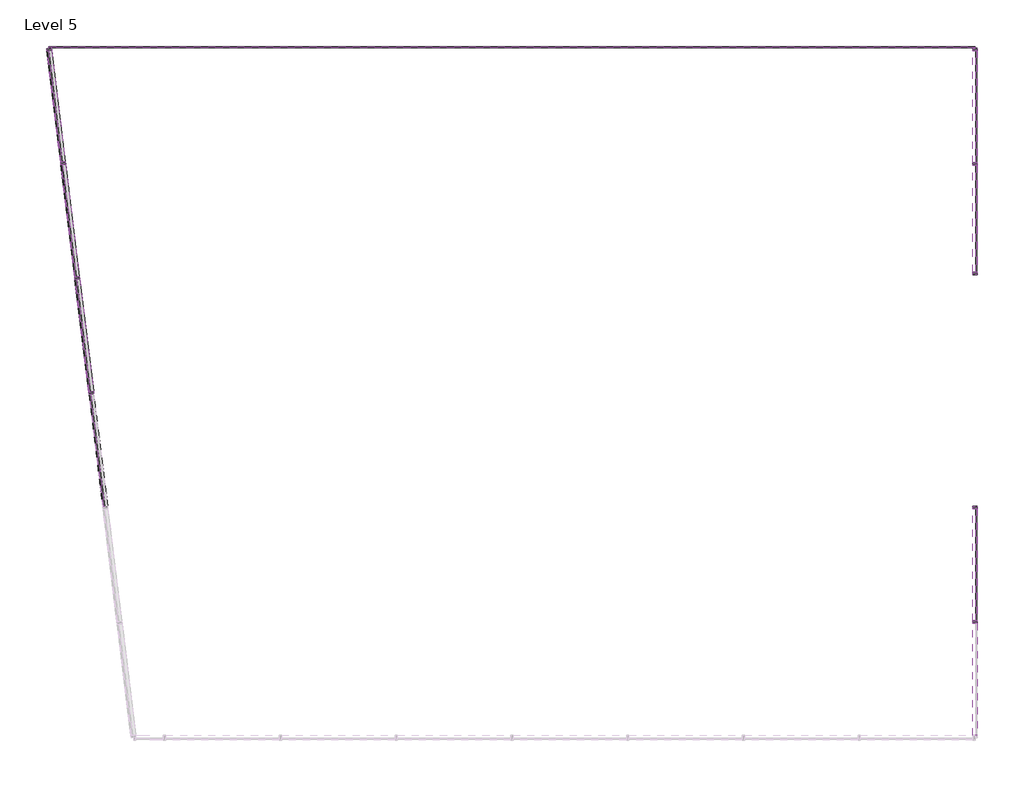
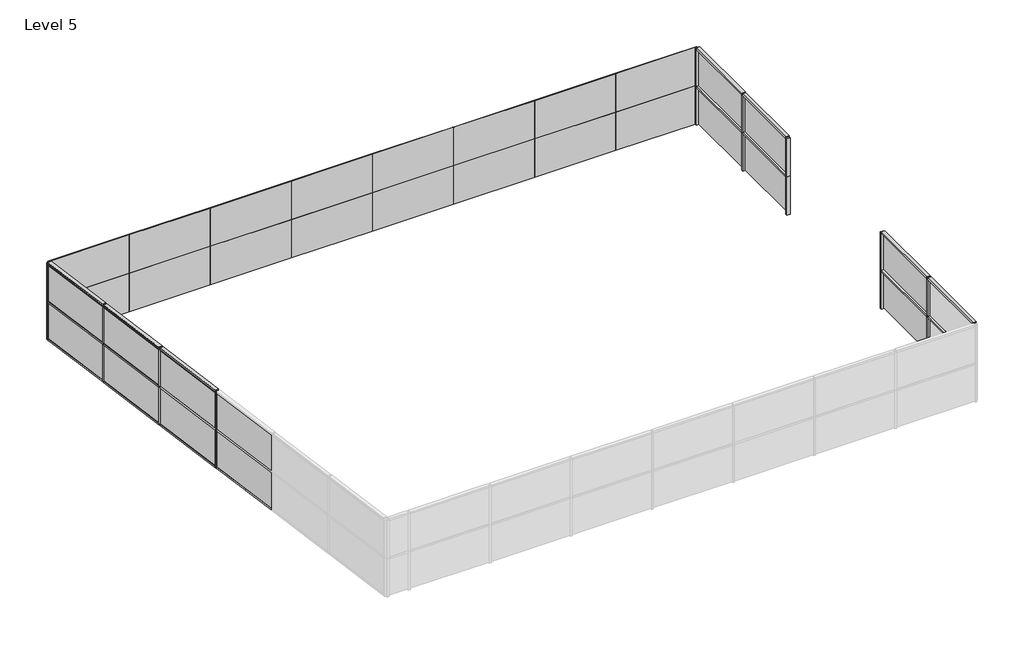
# One storey, part 2 of 2: 50 members, 38 plates.
"""IFC4 building model written with IfcOpenShell, lengths in millimetres."""

from ifc_helpers import new_model, si_unit, origin, place, context, project, spatial, transform, mapped, element, save
from components import member_71c27fd2, member_daa7a266, member_82905deb, member_19d0a4ec, member_8cef0660, member_db480205, member_4491d118, member_46bdb8c2, system_panel_glazed_1e57f9bb, system_panel_glazed_37f15d2e, system_panel_glazed_3620f98e, system_panel_glazed_e46d4b42, system_panel_glazed_2a6c68b7, system_panel_glazed_d483336f

model = new_model("IFC4")

# Units and contexts
model_context = context("Model", 3, world=origin())
ifc_project = project(units=[si_unit("LENGTHUNIT", "METRE", prefix="MILLI")], contexts=[model_context])

# Site, building, storey
site = spatial("IfcSite", under=ifc_project)
building = spatial("IfcBuilding", under=site)
storey = spatial("IfcBuildingStorey", under=building, Name="Level 5", Elevation=12192.0)

# Members
placement = place(None, origin())
member_shape = member_71c27fd2(model_context)
element("IfcMember", 1, ObjectType="Rectangular Mullion : 2.5\" x 5\" rectangular", at=placement, inside=storey, context=model_context, shape_type="MappedRepresentation", body=[
    mapped(member_shape, transform((-10473.7456604, 11109.5209701, 12192.0), x_axis=(0.0, 0.0, -1.0), y_axis=(-0.9925461516413222, -0.12186934340514603, 0.0), z_axis=(-0.12186934340514603, 0.9925461516413222, 0.0))),
])
member_2_shape = member_daa7a266(model_context)
element("IfcMember", 2, ObjectType="Rectangular Mullion : 2.5\" x 5\" rectangular", at=placement, inside=storey, context=model_context, shape_type="MappedRepresentation", body=[
    mapped(member_2_shape, transform((-10113.8959567, 8178.7803212, 15240.0), x_axis=(0.0, 0.0, 1.0), y_axis=(-0.9925461516413222, -0.12186934340514625, 0.0), z_axis=(0.12186934340514625, -0.9925461516413222, 0.0))),
])
member_3_shape = member_82905deb(model_context)
element("IfcMember", 3, ObjectType="Rectangular Mullion : 2.5\" x 5\" rectangular", at=placement, inside=storey, context=model_context, shape_type="MappedRepresentation", body=[
    mapped(member_3_shape, transform((-9367.1110876, 2096.7056405, 15240.0), x_axis=(-0.1218693434051459, 0.9925461516413222, 0.0), y_axis=(-0.9925461516413222, -0.1218693434051459, 0.0), z_axis=(0.0, 0.0, 1.0))),
])
element("IfcMember", 4, ObjectType="Rectangular Mullion : 2.5\" x 5\" rectangular", at=placement, inside=storey, context=model_context, shape_type="MappedRepresentation", body=[
    mapped(member_3_shape, transform((-9738.5688463, 5121.9863107, 15240.0), x_axis=(-0.1218693434051459, 0.9925461516413222, 0.0), y_axis=(-0.9925461516413222, -0.1218693434051459, 0.0), z_axis=(0.0, 0.0, 1.0))),
])
element("IfcMember", 5, ObjectType="Rectangular Mullion : 2.5\" x 5\" rectangular", at=placement, inside=storey, context=model_context, shape_type="MappedRepresentation", body=[
    mapped(member_3_shape, transform((-10110.026605, 8147.2669809, 15240.0), x_axis=(-0.1218693434051459, 0.9925461516413222, 0.0), y_axis=(-0.9925461516413222, -0.1218693434051459, 0.0), z_axis=(0.0, 0.0, 1.0))),
])
member_4_shape = member_19d0a4ec(model_context)
element("IfcMember", 6, ObjectType="Rectangular Mullion : 2.5\" x 5\" rectangular", at=placement, inside=storey, context=model_context, shape_type="MappedRepresentation", body=[
    mapped(member_4_shape, transform((-10113.8959567, 8178.7803212, 13716.0), x_axis=(0.0, 0.0, 1.0), y_axis=(-0.9925461516413222, -0.12186934340514609, 0.0), z_axis=(0.12186934340514609, -0.9925461516413222, 0.0))),
])
element("IfcMember", 7, ObjectType="Rectangular Mullion : 2.5\" x 5\" rectangular", at=placement, inside=storey, context=model_context, shape_type="MappedRepresentation", body=[
    mapped(member_4_shape, transform((-10113.8959567, 8178.7803212, 15240.0), x_axis=(0.0, 0.0, 1.0), y_axis=(-0.9925461516413223, -0.1218693434051454, 0.0), z_axis=(0.1218693434051454, -0.9925461516413223, 0.0))),
])
element("IfcMember", 8, ObjectType="Rectangular Mullion : 2.5\" x 5\" rectangular", at=placement, inside=storey, context=model_context, shape_type="MappedRepresentation", body=[
    mapped(member_4_shape, transform((-10113.8959567, 8178.7803212, 13716.0), x_axis=(0.0, 0.0, 1.0), y_axis=(-0.9925461516413223, -0.1218693434051456, 0.0), z_axis=(0.12186934340514559, -0.9925461516413222, 0.0))),
])
element("IfcMember", 9, ObjectType="Rectangular Mullion : 2.5\" x 5\" rectangular", at=placement, inside=storey, context=model_context, shape_type="MappedRepresentation", body=[
    mapped(member_4_shape, transform((13902.5156363, -946.6363705, 13716.0), x_axis=(0.0, 0.0, 1.0), y_axis=(1.0, 0.0, 0.0), z_axis=(0.0, 1.0, 0.0))),
])
element("IfcMember", 10, ObjectType="Rectangular Mullion : 2.5\" x 5\" rectangular", at=placement, inside=storey, context=model_context, shape_type="MappedRepresentation", body=[
    mapped(member_4_shape, transform((13902.5156363, -3962.8863708, 13716.0), x_axis=(0.0, 0.0, 1.0), y_axis=(1.0, 0.0, 0.0), z_axis=(0.0, 1.0, 0.0))),
])
element("IfcMember", 11, ObjectType="Rectangular Mullion : 2.5\" x 5\" rectangular", at=placement, inside=storey, context=model_context, shape_type="MappedRepresentation", body=[
    mapped(member_4_shape, transform((13902.5156363, -946.6363705, 15240.0), x_axis=(0.0, 0.0, 1.0), y_axis=(1.0, 0.0, 0.0), z_axis=(0.0, 1.0, 0.0))),
])
element("IfcMember", 12, ObjectType="Rectangular Mullion : 2.5\" x 5\" rectangular", at=placement, inside=storey, context=model_context, shape_type="MappedRepresentation", body=[
    mapped(member_4_shape, transform((13902.5156363, -3962.8863708, 15240.0), x_axis=(0.0, 0.0, 1.0), y_axis=(1.0, 0.0, 0.0), z_axis=(0.0, 1.0, 0.0))),
])
element("IfcMember", 13, ObjectType="Rectangular Mullion : 2.5\" x 5\" rectangular", at=placement, inside=storey, context=model_context, shape_type="MappedRepresentation", body=[
    mapped(member_4_shape, transform((13902.5156363, 11109.0476508, 13716.0), x_axis=(0.0, 0.0, 1.0), y_axis=(1.0, 0.0, 0.0), z_axis=(0.0, 1.0, 0.0))),
])
element("IfcMember", 14, ObjectType="Rectangular Mullion : 2.5\" x 5\" rectangular", at=placement, inside=storey, context=model_context, shape_type="MappedRepresentation", body=[
    mapped(member_4_shape, transform((13902.5156363, 11109.0476508, 15240.0), x_axis=(0.0, 0.0, 1.0), y_axis=(1.0, 0.0, 0.0), z_axis=(0.0, 1.0, 0.0))),
])
member_5_shape = member_8cef0660(model_context)
element("IfcMember", 15, ObjectType="Rectangular Mullion : 2.5\" x 5\" rectangular", at=placement, inside=storey, context=model_context, shape_type="MappedRepresentation", body=[
    mapped(member_5_shape, transform((-9370.9804393, 2128.2189808, 13716.0), x_axis=(0.0, 0.0, 1.0), y_axis=(-0.9925461516413222, -0.12186934340514592, 0.0), z_axis=(0.12186934340514592, -0.9925461516413222, 0.0))),
])
element("IfcMember", 16, ObjectType="Rectangular Mullion : 2.5\" x 5\" rectangular", at=placement, inside=storey, context=model_context, shape_type="MappedRepresentation", body=[
    mapped(member_5_shape, transform((-9742.438198, 5153.499651, 13716.0), x_axis=(0.0, 0.0, 1.0), y_axis=(-0.9925461516413222, -0.1218693434051457, 0.0), z_axis=(0.1218693434051457, -0.9925461516413222, 0.0))),
])
element("IfcMember", 17, ObjectType="Rectangular Mullion : 2.5\" x 5\" rectangular", at=placement, inside=storey, context=model_context, shape_type="MappedRepresentation", body=[
    mapped(member_5_shape, transform((-9370.9804393, 2128.2189808, 15240.0), x_axis=(0.0, 0.0, 1.0), y_axis=(-0.9925461516413222, -0.12186934340514592, 0.0), z_axis=(0.12186934340514592, -0.9925461516413222, 0.0))),
])
element("IfcMember", 18, ObjectType="Rectangular Mullion : 2.5\" x 5\" rectangular", at=placement, inside=storey, context=model_context, shape_type="MappedRepresentation", body=[
    mapped(member_5_shape, transform((-9742.438198, 5153.499651, 15240.0), x_axis=(0.0, 0.0, 1.0), y_axis=(-0.9925461516413222, -0.12186934340514606, 0.0), z_axis=(0.12186934340514606, -0.9925461516413222, 0.0))),
])
element("IfcMember", 19, ObjectType="Rectangular Mullion : 2.5\" x 5\" rectangular", at=placement, inside=storey, context=model_context, shape_type="MappedRepresentation", body=[
    mapped(member_5_shape, transform((-9370.9804393, 2128.2189808, 13716.0), x_axis=(0.0, 0.0, 1.0), y_axis=(-0.9925461516413222, -0.12186934340514592, 0.0), z_axis=(0.12186934340514592, -0.9925461516413222, 0.0))),
])
element("IfcMember", 20, ObjectType="Rectangular Mullion : 2.5\" x 5\" rectangular", at=placement, inside=storey, context=model_context, shape_type="MappedRepresentation", body=[
    mapped(member_5_shape, transform((-9742.438198, 5153.499651, 13716.0), x_axis=(0.0, 0.0, 1.0), y_axis=(-0.9925461516413222, -0.12186934340514602, 0.0), z_axis=(0.12186934340514602, -0.9925461516413222, 0.0))),
])
member_6_shape = member_db480205(model_context)
element("IfcMember", 21, ObjectType="Rectangular Mullion : 2.5\" x 5\" rectangular", at=placement, inside=storey, context=model_context, shape_type="MappedRepresentation", body=[
    mapped(member_6_shape, transform((-9363.241736, 2065.1923001, 12192.0), x_axis=(0.0, 0.0, -1.0), y_axis=(-0.9925461516413222, -0.12186934340514602, 0.0), z_axis=(-0.12186934340514602, 0.9925461516413222, 0.0))),
])
element("IfcMember", 22, ObjectType="Rectangular Mullion : 2.5\" x 5\" rectangular", at=placement, inside=storey, context=model_context, shape_type="MappedRepresentation", body=[
    mapped(member_6_shape, transform((-9734.6994947, 5090.4729703, 12192.0), x_axis=(0.0, 0.0, -1.0), y_axis=(-0.9925461516413223, -0.12186934340514559, 0.0), z_axis=(-0.12186934340514559, 0.9925461516413223, 0.0))),
])
element("IfcMember", 23, ObjectType="Rectangular Mullion : 2.5\" x 5\" rectangular", at=placement, inside=storey, context=model_context, shape_type="MappedRepresentation", body=[
    mapped(member_6_shape, transform((-10106.1572534, 8115.7536405, 12192.0), x_axis=(0.0, 0.0, -1.0), y_axis=(-0.9925461516413222, -0.1218693434051461, 0.0), z_axis=(-0.1218693434051461, 0.9925461516413222, 0.0))),
])
element("IfcMember", 24, ObjectType="Rectangular Mullion : 2.5\" x 5\" rectangular", at=placement, inside=storey, context=model_context, shape_type="MappedRepresentation", body=[
    mapped(member_6_shape, transform((-9370.9804393, 2128.2189808, 15240.0), x_axis=(0.0, 0.0, 1.0), y_axis=(-0.9925461516413222, -0.12186934340514592, 0.0), z_axis=(0.12186934340514592, -0.9925461516413222, 0.0))),
])
element("IfcMember", 25, ObjectType="Rectangular Mullion : 2.5\" x 5\" rectangular", at=placement, inside=storey, context=model_context, shape_type="MappedRepresentation", body=[
    mapped(member_6_shape, transform((-9742.438198, 5153.499651, 15240.0), x_axis=(0.0, 0.0, 1.0), y_axis=(-0.9925461516413222, -0.1218693434051457, 0.0), z_axis=(0.1218693434051457, -0.9925461516413222, 0.0))),
])
element("IfcMember", 26, ObjectType="Rectangular Mullion : 2.5\" x 5\" rectangular", at=placement, inside=storey, context=model_context, shape_type="MappedRepresentation", body=[
    mapped(member_3_shape, transform((-9367.1110876, 2096.7056405, 13716.0), x_axis=(-0.1218693434051459, 0.9925461516413222, 0.0), y_axis=(-0.9925461516413222, -0.1218693434051459, 0.0), z_axis=(0.0, 0.0, 1.0))),
])
element("IfcMember", 27, ObjectType="Rectangular Mullion : 2.5\" x 5\" rectangular", at=placement, inside=storey, context=model_context, shape_type="MappedRepresentation", body=[
    mapped(member_3_shape, transform((-9738.5688463, 5121.9863107, 13716.0), x_axis=(-0.1218693434051459, 0.9925461516413222, 0.0), y_axis=(-0.9925461516413222, -0.1218693434051459, 0.0), z_axis=(0.0, 0.0, 1.0))),
])
element("IfcMember", 28, ObjectType="Rectangular Mullion : 2.5\" x 5\" rectangular", at=placement, inside=storey, context=model_context, shape_type="MappedRepresentation", body=[
    mapped(member_3_shape, transform((-10110.026605, 8147.2669809, 13716.0), x_axis=(-0.1218693434051459, 0.9925461516413222, 0.0), y_axis=(-0.9925461516413222, -0.1218693434051459, 0.0), z_axis=(0.0, 0.0, 1.0))),
])
element("IfcMember", 29, ObjectType="Rectangular Mullion : 2.5\" x 5\" rectangular", at=placement, inside=storey, context=model_context, shape_type="MappedRepresentation", body=[
    mapped(member_3_shape, transform((-9367.1110876, 2096.7056405, 15240.0), x_axis=(-0.1218693434051459, 0.9925461516413222, 0.0), y_axis=(-0.9925461516413222, -0.1218693434051459, 0.0), z_axis=(0.0, 0.0, 1.0))),
])
element("IfcMember", 30, ObjectType="Rectangular Mullion : 2.5\" x 5\" rectangular", at=placement, inside=storey, context=model_context, shape_type="MappedRepresentation", body=[
    mapped(member_3_shape, transform((-9738.5688463, 5121.9863107, 15240.0), x_axis=(-0.1218693434051459, 0.9925461516413222, 0.0), y_axis=(-0.9925461516413222, -0.1218693434051459, 0.0), z_axis=(0.0, 0.0, 1.0))),
])
element("IfcMember", 31, ObjectType="Rectangular Mullion : 2.5\" x 5\" rectangular", at=placement, inside=storey, context=model_context, shape_type="MappedRepresentation", body=[
    mapped(member_3_shape, transform((-10110.026605, 8147.2669809, 15240.0), x_axis=(-0.1218693434051459, 0.9925461516413222, 0.0), y_axis=(-0.9925461516413222, -0.1218693434051459, 0.0), z_axis=(0.0, 0.0, 1.0))),
])
element("IfcMember", 32, ObjectType="Rectangular Mullion : 2.5\" x 5\" rectangular", at=placement, inside=storey, context=model_context, shape_type="MappedRepresentation", body=[
    mapped(member_3_shape, transform((-9367.1110876, 2096.7056405, 13716.0), x_axis=(-0.1218693434051459, 0.9925461516413222, 0.0), y_axis=(-0.9925461516413222, -0.1218693434051459, 0.0), z_axis=(0.0, 0.0, 1.0))),
])
element("IfcMember", 33, ObjectType="Rectangular Mullion : 2.5\" x 5\" rectangular", at=placement, inside=storey, context=model_context, shape_type="MappedRepresentation", body=[
    mapped(member_3_shape, transform((-9738.5688463, 5121.9863107, 13716.0), x_axis=(-0.1218693434051459, 0.9925461516413222, 0.0), y_axis=(-0.9925461516413222, -0.1218693434051459, 0.0), z_axis=(0.0, 0.0, 1.0))),
])
element("IfcMember", 34, ObjectType="Rectangular Mullion : 2.5\" x 5\" rectangular", at=placement, inside=storey, context=model_context, shape_type="MappedRepresentation", body=[
    mapped(member_3_shape, transform((-10110.026605, 8147.2669809, 13716.0), x_axis=(-0.1218693434051459, 0.9925461516413222, 0.0), y_axis=(-0.9925461516413222, -0.1218693434051459, 0.0), z_axis=(0.0, 0.0, 1.0))),
])
element("IfcMember", 35, ObjectType="Rectangular Mullion : 2.5\" x 5\" rectangular", at=placement, inside=storey, context=model_context, shape_type="MappedRepresentation", body=[
    mapped(member_3_shape, transform((13902.5156363, -3931.1363708, 13716.0), x_axis=(0.0, -1.0, 0.0), y_axis=(1.0, 0.0, 0.0), z_axis=(0.0, 0.0, 1.0))),
])
element("IfcMember", 36, ObjectType="Rectangular Mullion : 2.5\" x 5\" rectangular", at=placement, inside=storey, context=model_context, shape_type="MappedRepresentation", body=[
    mapped(member_3_shape, transform((13902.5156363, -3931.1363708, 15240.0), x_axis=(0.0, -1.0, 0.0), y_axis=(1.0, 0.0, 0.0), z_axis=(0.0, 0.0, 1.0))),
])
element("IfcMember", 37, ObjectType="Rectangular Mullion : 2.5\" x 5\" rectangular", at=placement, inside=storey, context=model_context, shape_type="MappedRepresentation", body=[
    mapped(member_3_shape, transform((13902.5156363, 8124.5476505, 13716.0), x_axis=(0.0, -1.0, 0.0), y_axis=(1.0, 0.0, 0.0), z_axis=(0.0, 0.0, 1.0))),
])
element("IfcMember", 38, ObjectType="Rectangular Mullion : 2.5\" x 5\" rectangular", at=placement, inside=storey, context=model_context, shape_type="MappedRepresentation", body=[
    mapped(member_3_shape, transform((13902.5156363, 8124.5476505, 15240.0), x_axis=(0.0, -1.0, 0.0), y_axis=(1.0, 0.0, 0.0), z_axis=(0.0, 0.0, 1.0))),
])
member_7_shape = member_4491d118(model_context)
element("IfcMember", 39, ObjectType="Rectangular Mullion : 2.5\" x 5\" rectangular", at=placement, inside=storey, context=model_context, shape_type="MappedRepresentation", body=[
    mapped(member_7_shape, transform((-10481.4843637, 11172.5476508, 15240.0), x_axis=(-0.1218693434051459, 0.9925461516413222, 0.0), y_axis=(-0.9925461516413222, -0.1218693434051459, 0.0), z_axis=(0.0, 0.0, 1.0))),
])
element("IfcMember", 40, ObjectType="Rectangular Mullion : 2.5\" x 5\" rectangular", at=placement, inside=storey, context=model_context, shape_type="MappedRepresentation", body=[
    mapped(member_7_shape, transform((13902.5156363, -883.1363705, 12192.0), x_axis=(0.0, 1.0, 0.0), y_axis=(1.0, 0.0, 0.0), z_axis=(0.0, 0.0, -1.0))),
])
element("IfcMember", 41, ObjectType="Rectangular Mullion : 2.5\" x 5\" rectangular", at=placement, inside=storey, context=model_context, shape_type="MappedRepresentation", body=[
    mapped(member_7_shape, transform((13902.5156363, -883.1363705, 13716.0), x_axis=(0.0, 1.0, 0.0), y_axis=(1.0, 0.0, 0.0), z_axis=(0.0, 0.0, -1.0))),
])
element("IfcMember", 42, ObjectType="Rectangular Mullion : 2.5\" x 5\" rectangular", at=placement, inside=storey, context=model_context, shape_type="MappedRepresentation", body=[
    mapped(member_7_shape, transform((13902.5156363, 11172.5476508, 12192.0), x_axis=(0.0, 1.0, 0.0), y_axis=(1.0, 0.0, 0.0), z_axis=(0.0, 0.0, -1.0))),
])
element("IfcMember", 43, ObjectType="Rectangular Mullion : 2.5\" x 5\" rectangular", at=placement, inside=storey, context=model_context, shape_type="MappedRepresentation", body=[
    mapped(member_7_shape, transform((13902.5156363, 11172.5476508, 13716.0), x_axis=(0.0, 1.0, 0.0), y_axis=(1.0, 0.0, 0.0), z_axis=(0.0, 0.0, -1.0))),
])
element("IfcMember", 44, ObjectType="Rectangular Mullion : 2.5\" x 5\" rectangular", at=placement, inside=storey, context=model_context, shape_type="MappedRepresentation", body=[
    mapped(member_7_shape, transform((-10481.4843637, 11172.5476508, 13716.0), x_axis=(-0.1218693434051459, 0.9925461516413222, 0.0), y_axis=(-0.9925461516413222, -0.1218693434051459, 0.0), z_axis=(0.0, 0.0, 1.0))),
])
element("IfcMember", 45, ObjectType="Rectangular Mullion : 2.5\" x 5\" rectangular", at=placement, inside=storey, context=model_context, shape_type="MappedRepresentation", body=[
    mapped(member_7_shape, transform((-10481.4843637, 11172.5476508, 15240.0), x_axis=(-0.1218693434051459, 0.9925461516413222, 0.0), y_axis=(-0.9925461516413222, -0.1218693434051459, 0.0), z_axis=(0.0, 0.0, 1.0))),
])
element("IfcMember", 46, ObjectType="Rectangular Mullion : 2.5\" x 5\" rectangular", at=placement, inside=storey, context=model_context, shape_type="MappedRepresentation", body=[
    mapped(member_7_shape, transform((-10481.4843637, 11172.5476508, 13716.0), x_axis=(-0.1218693434051459, 0.9925461516413222, 0.0), y_axis=(-0.9925461516413222, -0.1218693434051459, 0.0), z_axis=(0.0, 0.0, 1.0))),
])
element("IfcMember", 47, ObjectType="Rectangular Mullion : 2.5\" x 5\" rectangular", at=placement, inside=storey, context=model_context, shape_type="MappedRepresentation", body=[
    mapped(member_7_shape, transform((13902.5156363, 5212.8636295, 13716.0), x_axis=(0.0, -1.0, 0.0), y_axis=(1.0, 0.0, 0.0), z_axis=(0.0, 0.0, 1.0))),
])
element("IfcMember", 48, ObjectType="Rectangular Mullion : 2.5\" x 5\" rectangular", at=placement, inside=storey, context=model_context, shape_type="MappedRepresentation", body=[
    mapped(member_7_shape, transform((13902.5156363, 5212.8636295, 15240.0), x_axis=(0.0, -1.0, 0.0), y_axis=(1.0, 0.0, 0.0), z_axis=(0.0, 0.0, 1.0))),
])
member_8_shape = member_46bdb8c2(model_context)
element("IfcMember", 49, ObjectType="Rectangular Mullion : 2.5\" x 5\" rectangular", at=placement, inside=storey, context=model_context, shape_type="MappedRepresentation", body=[
    mapped(member_8_shape, transform((13902.5156363, 8092.7976505, 13716.0), x_axis=(0.0, 0.0, 1.0), y_axis=(1.0, 0.0, 0.0), z_axis=(0.0, 1.0, 0.0))),
])
element("IfcMember", 50, ObjectType="Rectangular Mullion : 2.5\" x 5\" rectangular", at=placement, inside=storey, context=model_context, shape_type="MappedRepresentation", body=[
    mapped(member_8_shape, transform((13902.5156363, 8092.7976505, 15240.0), x_axis=(0.0, 0.0, 1.0), y_axis=(1.0, 0.0, 0.0), z_axis=(0.0, 1.0, 0.0))),
])

# Plates
system_panel_glazed_shape = system_panel_glazed_1e57f9bb(model_context)
element("IfcPlate", 51, ObjectType="System Panel : Glazed", at=placement, inside=storey, context=model_context, shape_type="MappedRepresentation", body=[
    mapped(system_panel_glazed_shape, transform((-8957.4843636, 11172.5476508, 12192.0), x_axis=(1.0, 0.0, 0.0), y_axis=(0.0, 1.0, 0.0), z_axis=(0.0, 0.0, 1.0))),
])
element("IfcPlate", 52, ObjectType="System Panel : Glazed", at=placement, inside=storey, context=model_context, shape_type="MappedRepresentation", body=[
    mapped(system_panel_glazed_shape, transform((-5909.4843634, 11172.5476508, 12192.0), x_axis=(1.0, 0.0, 0.0), y_axis=(0.0, 1.0, 0.0), z_axis=(0.0, 0.0, 1.0))),
])
element("IfcPlate", 53, ObjectType="System Panel : Glazed", at=placement, inside=storey, context=model_context, shape_type="MappedRepresentation", body=[
    mapped(system_panel_glazed_shape, transform((-2861.4843634, 11172.5476508, 12192.0), x_axis=(1.0, 0.0, 0.0), y_axis=(0.0, 1.0, 0.0), z_axis=(0.0, 0.0, 1.0))),
])
element("IfcPlate", 54, ObjectType="System Panel : Glazed", at=placement, inside=storey, context=model_context, shape_type="MappedRepresentation", body=[
    mapped(system_panel_glazed_shape, transform((186.5156366, 11172.5476508, 12192.0), x_axis=(1.0, 0.0, 0.0), y_axis=(0.0, 1.0, 0.0), z_axis=(0.0, 0.0, 1.0))),
])
element("IfcPlate", 55, ObjectType="System Panel : Glazed", at=placement, inside=storey, context=model_context, shape_type="MappedRepresentation", body=[
    mapped(system_panel_glazed_shape, transform((3234.5156366, 11172.5476508, 12192.0), x_axis=(1.0, 0.0, 0.0), y_axis=(0.0, 1.0, 0.0), z_axis=(0.0, 0.0, 1.0))),
])
element("IfcPlate", 56, ObjectType="System Panel : Glazed", at=placement, inside=storey, context=model_context, shape_type="MappedRepresentation", body=[
    mapped(system_panel_glazed_shape, transform((6282.5156366, 11172.5476508, 12192.0), x_axis=(1.0, 0.0, 0.0), y_axis=(0.0, 1.0, 0.0), z_axis=(0.0, 0.0, 1.0))),
])
element("IfcPlate", 57, ObjectType="System Panel : Glazed", at=placement, inside=storey, context=model_context, shape_type="MappedRepresentation", body=[
    mapped(system_panel_glazed_shape, transform((9330.5156366, 11172.5476508, 12192.0), x_axis=(1.0, 0.0, 0.0), y_axis=(0.0, 1.0, 0.0), z_axis=(0.0, 0.0, 1.0))),
])
element("IfcPlate", 58, ObjectType="System Panel : Glazed", at=placement, inside=storey, context=model_context, shape_type="MappedRepresentation", body=[
    mapped(system_panel_glazed_shape, transform((12378.5156364, 11172.5476508, 12192.0), x_axis=(1.0, 0.0, 0.0), y_axis=(0.0, 1.0, 0.0), z_axis=(0.0, 0.0, 1.0))),
])
element("IfcPlate", 59, ObjectType="System Panel : Glazed", at=placement, inside=storey, context=model_context, shape_type="MappedRepresentation", body=[
    mapped(system_panel_glazed_shape, transform((-8957.4843636, 11172.5476508, 13716.0), x_axis=(1.0, 0.0, 0.0), y_axis=(0.0, 1.0, 0.0), z_axis=(0.0, 0.0, 1.0))),
])
element("IfcPlate", 60, ObjectType="System Panel : Glazed", at=placement, inside=storey, context=model_context, shape_type="MappedRepresentation", body=[
    mapped(system_panel_glazed_shape, transform((-5909.4843634, 11172.5476508, 13716.0), x_axis=(1.0, 0.0, 0.0), y_axis=(0.0, 1.0, 0.0), z_axis=(0.0, 0.0, 1.0))),
])
element("IfcPlate", 61, ObjectType="System Panel : Glazed", at=placement, inside=storey, context=model_context, shape_type="MappedRepresentation", body=[
    mapped(system_panel_glazed_shape, transform((-2861.4843634, 11172.5476508, 13716.0), x_axis=(1.0, 0.0, 0.0), y_axis=(0.0, 1.0, 0.0), z_axis=(0.0, 0.0, 1.0))),
])
element("IfcPlate", 62, ObjectType="System Panel : Glazed", at=placement, inside=storey, context=model_context, shape_type="MappedRepresentation", body=[
    mapped(system_panel_glazed_shape, transform((186.5156366, 11172.5476508, 13716.0), x_axis=(1.0, 0.0, 0.0), y_axis=(0.0, 1.0, 0.0), z_axis=(0.0, 0.0, 1.0))),
])
element("IfcPlate", 63, ObjectType="System Panel : Glazed", at=placement, inside=storey, context=model_context, shape_type="MappedRepresentation", body=[
    mapped(system_panel_glazed_shape, transform((3234.5156366, 11172.5476508, 13716.0), x_axis=(1.0, 0.0, 0.0), y_axis=(0.0, 1.0, 0.0), z_axis=(0.0, 0.0, 1.0))),
])
element("IfcPlate", 64, ObjectType="System Panel : Glazed", at=placement, inside=storey, context=model_context, shape_type="MappedRepresentation", body=[
    mapped(system_panel_glazed_shape, transform((6282.5156366, 11172.5476508, 13716.0), x_axis=(1.0, 0.0, 0.0), y_axis=(0.0, 1.0, 0.0), z_axis=(0.0, 0.0, 1.0))),
])
element("IfcPlate", 65, ObjectType="System Panel : Glazed", at=placement, inside=storey, context=model_context, shape_type="MappedRepresentation", body=[
    mapped(system_panel_glazed_shape, transform((9330.5156366, 11172.5476508, 13716.0), x_axis=(1.0, 0.0, 0.0), y_axis=(0.0, 1.0, 0.0), z_axis=(0.0, 0.0, 1.0))),
])
element("IfcPlate", 66, ObjectType="System Panel : Glazed", at=placement, inside=storey, context=model_context, shape_type="MappedRepresentation", body=[
    mapped(system_panel_glazed_shape, transform((12378.5156364, 11172.5476508, 13716.0), x_axis=(1.0, 0.0, 0.0), y_axis=(0.0, 1.0, 0.0), z_axis=(0.0, 0.0, 1.0))),
])
system_panel_glazed_2_shape = system_panel_glazed_37f15d2e(model_context)
element("IfcPlate", 67, ObjectType="System Panel : Glazed", at=placement, inside=storey, context=model_context, shape_type="MappedRepresentation", body=[
    mapped(system_panel_glazed_2_shape, transform((-10293.8208085, 9644.1506457, 13747.75), x_axis=(-0.1218693434051459, 0.9925461516413222, 0.0), y_axis=(-0.9925461516413222, -0.1218693434051459, 0.0), z_axis=(0.0, 0.0, 1.0))),
])
element("IfcPlate", 68, ObjectType="System Panel : Glazed", at=placement, inside=storey, context=model_context, shape_type="MappedRepresentation", body=[
    mapped(system_panel_glazed_2_shape, transform((-10293.8208085, 9644.1506457, 12255.5), x_axis=(-0.1218693434051459, 0.9925461516413222, 0.0), y_axis=(-0.9925461516413222, -0.1218693434051459, 0.0), z_axis=(0.0, 0.0, 1.0))),
])
system_panel_glazed_3_shape = system_panel_glazed_3620f98e(model_context)
element("IfcPlate", 69, ObjectType="System Panel : Glazed", at=placement, inside=storey, context=model_context, shape_type="MappedRepresentation", body=[
    mapped(system_panel_glazed_3_shape, transform((-9181.3822083, 584.0653054, 13747.75), x_axis=(-0.1218693434051459, 0.9925461516413222, 0.0), y_axis=(-0.9925461516413222, -0.1218693434051459, 0.0), z_axis=(0.0, 0.0, 1.0))),
])
element("IfcPlate", 70, ObjectType="System Panel : Glazed", at=placement, inside=storey, context=model_context, shape_type="MappedRepresentation", body=[
    mapped(system_panel_glazed_3_shape, transform((-9552.839967, 3609.3459756, 13747.75), x_axis=(-0.1218693434051459, 0.9925461516413222, 0.0), y_axis=(-0.9925461516413222, -0.1218693434051459, 0.0), z_axis=(0.0, 0.0, 1.0))),
])
element("IfcPlate", 71, ObjectType="System Panel : Glazed", at=placement, inside=storey, context=model_context, shape_type="MappedRepresentation", body=[
    mapped(system_panel_glazed_3_shape, transform((-9924.2977257, 6634.6266458, 13747.75), x_axis=(-0.1218693434051459, 0.9925461516413222, 0.0), y_axis=(-0.9925461516413222, -0.1218693434051459, 0.0), z_axis=(0.0, 0.0, 1.0))),
])
element("IfcPlate", 72, ObjectType="System Panel : Glazed", at=placement, inside=storey, context=model_context, shape_type="MappedRepresentation", body=[
    mapped(system_panel_glazed_3_shape, transform((-9181.3822083, 584.0653054, 12255.5), x_axis=(-0.1218693434051459, 0.9925461516413222, 0.0), y_axis=(-0.9925461516413222, -0.1218693434051459, 0.0), z_axis=(0.0, 0.0, 1.0))),
])
element("IfcPlate", 73, ObjectType="System Panel : Glazed", at=placement, inside=storey, context=model_context, shape_type="MappedRepresentation", body=[
    mapped(system_panel_glazed_3_shape, transform((-9552.839967, 3609.3459756, 12255.5), x_axis=(-0.1218693434051459, 0.9925461516413222, 0.0), y_axis=(-0.9925461516413222, -0.1218693434051459, 0.0), z_axis=(0.0, 0.0, 1.0))),
])
element("IfcPlate", 74, ObjectType="System Panel : Glazed", at=placement, inside=storey, context=model_context, shape_type="MappedRepresentation", body=[
    mapped(system_panel_glazed_3_shape, transform((-9924.2977257, 6634.6266458, 12255.5), x_axis=(-0.1218693434051459, 0.9925461516413222, 0.0), y_axis=(-0.9925461516413222, -0.1218693434051459, 0.0), z_axis=(0.0, 0.0, 1.0))),
])
system_panel_glazed_4_shape = system_panel_glazed_e46d4b42(model_context)
element("IfcPlate", 75, ObjectType="System Panel : Glazed", at=placement, inside=storey, context=model_context, shape_type="MappedRepresentation", body=[
    mapped(system_panel_glazed_4_shape, transform((-10293.8208085, 9644.1506457, 12223.75), x_axis=(-0.1218693434051459, 0.9925461516413222, 0.0), y_axis=(-0.9925461516413222, -0.1218693434051459, 0.0), z_axis=(0.0, 0.0, 1.0))),
])
element("IfcPlate", 76, ObjectType="System Panel : Glazed", at=placement, inside=storey, context=model_context, shape_type="MappedRepresentation", body=[
    mapped(system_panel_glazed_4_shape, transform((13902.5156363, -2423.0113706, 12223.75), x_axis=(0.0, -1.0, 0.0), y_axis=(1.0, 0.0, 0.0), z_axis=(0.0, 0.0, 1.0))),
])
element("IfcPlate", 77, ObjectType="System Panel : Glazed", at=placement, inside=storey, context=model_context, shape_type="MappedRepresentation", body=[
    mapped(system_panel_glazed_4_shape, transform((13902.5156363, -2423.0113706, 13747.75), x_axis=(0.0, -1.0, 0.0), y_axis=(1.0, 0.0, 0.0), z_axis=(0.0, 0.0, 1.0))),
])
element("IfcPlate", 78, ObjectType="System Panel : Glazed", at=placement, inside=storey, context=model_context, shape_type="MappedRepresentation", body=[
    mapped(system_panel_glazed_4_shape, transform((13902.5156363, 9632.6726506, 12223.75), x_axis=(0.0, -1.0, 0.0), y_axis=(1.0, 0.0, 0.0), z_axis=(0.0, 0.0, 1.0))),
])
element("IfcPlate", 79, ObjectType="System Panel : Glazed", at=placement, inside=storey, context=model_context, shape_type="MappedRepresentation", body=[
    mapped(system_panel_glazed_4_shape, transform((13902.5156363, 9632.6726506, 13747.75), x_axis=(0.0, -1.0, 0.0), y_axis=(1.0, 0.0, 0.0), z_axis=(0.0, 0.0, 1.0))),
])
element("IfcPlate", 80, ObjectType="System Panel : Glazed", at=placement, inside=storey, context=model_context, shape_type="MappedRepresentation", body=[
    mapped(system_panel_glazed_4_shape, transform((-10293.8208085, 9644.1506457, 13747.75), x_axis=(-0.1218693434051459, 0.9925461516413222, 0.0), y_axis=(-0.9925461516413222, -0.1218693434051459, 0.0), z_axis=(0.0, 0.0, 1.0))),
])
system_panel_glazed_5_shape = system_panel_glazed_2a6c68b7(model_context)
element("IfcPlate", 81, ObjectType="System Panel : Glazed", at=placement, inside=storey, context=model_context, shape_type="MappedRepresentation", body=[
    mapped(system_panel_glazed_5_shape, transform((-9181.3822083, 584.0653054, 12223.75), x_axis=(-0.1218693434051459, 0.9925461516413222, 0.0), y_axis=(-0.9925461516413222, -0.1218693434051459, 0.0), z_axis=(0.0, 0.0, 1.0))),
])
element("IfcPlate", 82, ObjectType="System Panel : Glazed", at=placement, inside=storey, context=model_context, shape_type="MappedRepresentation", body=[
    mapped(system_panel_glazed_5_shape, transform((-9552.839967, 3609.3459756, 12223.75), x_axis=(-0.1218693434051459, 0.9925461516413222, 0.0), y_axis=(-0.9925461516413222, -0.1218693434051459, 0.0), z_axis=(0.0, 0.0, 1.0))),
])
element("IfcPlate", 83, ObjectType="System Panel : Glazed", at=placement, inside=storey, context=model_context, shape_type="MappedRepresentation", body=[
    mapped(system_panel_glazed_5_shape, transform((-9924.2977257, 6634.6266458, 12223.75), x_axis=(-0.1218693434051459, 0.9925461516413222, 0.0), y_axis=(-0.9925461516413222, -0.1218693434051459, 0.0), z_axis=(0.0, 0.0, 1.0))),
])
element("IfcPlate", 84, ObjectType="System Panel : Glazed", at=placement, inside=storey, context=model_context, shape_type="MappedRepresentation", body=[
    mapped(system_panel_glazed_5_shape, transform((-9181.3822083, 584.0653054, 13747.75), x_axis=(-0.1218693434051459, 0.9925461516413222, 0.0), y_axis=(-0.9925461516413222, -0.1218693434051459, 0.0), z_axis=(0.0, 0.0, 1.0))),
])
element("IfcPlate", 85, ObjectType="System Panel : Glazed", at=placement, inside=storey, context=model_context, shape_type="MappedRepresentation", body=[
    mapped(system_panel_glazed_5_shape, transform((-9552.839967, 3609.3459756, 13747.75), x_axis=(-0.1218693434051459, 0.9925461516413222, 0.0), y_axis=(-0.9925461516413222, -0.1218693434051459, 0.0), z_axis=(0.0, 0.0, 1.0))),
])
element("IfcPlate", 86, ObjectType="System Panel : Glazed", at=placement, inside=storey, context=model_context, shape_type="MappedRepresentation", body=[
    mapped(system_panel_glazed_5_shape, transform((-9924.2977257, 6634.6266458, 13747.75), x_axis=(-0.1218693434051459, 0.9925461516413222, 0.0), y_axis=(-0.9925461516413222, -0.1218693434051459, 0.0), z_axis=(0.0, 0.0, 1.0))),
])
system_panel_glazed_6_shape = system_panel_glazed_d483336f(model_context)
element("IfcPlate", 87, ObjectType="System Panel : Glazed", at=placement, inside=storey, context=model_context, shape_type="MappedRepresentation", body=[
    mapped(system_panel_glazed_6_shape, transform((13902.5156363, 6684.58064, 12223.75), x_axis=(0.0, -1.0, 0.0), y_axis=(1.0, 0.0, 0.0), z_axis=(0.0, 0.0, 1.0))),
])
element("IfcPlate", 88, ObjectType="System Panel : Glazed", at=placement, inside=storey, context=model_context, shape_type="MappedRepresentation", body=[
    mapped(system_panel_glazed_6_shape, transform((13902.5156363, 6684.58064, 13747.75), x_axis=(0.0, -1.0, 0.0), y_axis=(1.0, 0.0, 0.0), z_axis=(0.0, 0.0, 1.0))),
])

save(model, "model.ifc")

# Revit data of these elements
# Type "Rectangular Mullion : 2.5\" x 5\" rectangular"
#   built-in parameter 1007304 = 0.416667 (stored number, unit not read)
#   built-in parameter 1007301 = 0.104167 (stored number, unit not read)
#   built-in parameter 1007300 = 0.104167 (stored number, unit not read)
# Type "System Panel : Glazed"
#   Construction Type Id = "GSP4R"
#   Analytic Construction = "1/8 in Pilkington single glazing"
#   Visual Light Transmittance = 0.9
#   Solar Heat Gain Coefficient = 0.86
#   Heat Transfer Coefficient (U) = 1.18115 BTU/(h·ft²·°F)
#   Define Thermal Properties by = 1
# Elements 1, 2, 3, 4, 5, 6, 7, 8, 9, 10, 11, 12, 13, 14, 15, 16, 17, 18, 19, 20, 21, 22, 23, 24, 25, 26, 27, 28, 29, 30, 31, 32, 33, 34, 35, 36, 37, 38, 39, 40, 41, 42, 43, 44, 45, 46, 47, 48, 49, 50 (IfcMember, "Rectangular Mullion : 2.5\" x 5\" rectangular")
#   Phase Created = New Construction
#   Materials on its faces: "Aluminum"
# Elements 51, 52, 53, 54, 55, 56, 57, 58, 59, 60, 61, 62, 63, 64, 65, 66, 67, 68, 69, 70, 71, 72, 73, 74, 75, 76, 77, 78, 79, 80, 81, 82, 83, 84, 85, 86, 87, 88 (IfcPlate, "System Panel : Glazed")
#   Phase Created = New Construction
#   Materials on its faces: "Glass"
# Materials
#   "Aluminum": class "Metal", colour RGB 247 247 247, transparency 0, Description = "Aluminum 6061", Cost = 0
#   "Glass": class "Glass", colour RGB 0 128 192, transparency 0.75, Description = "Soda Lime Glass", Cost = 0
